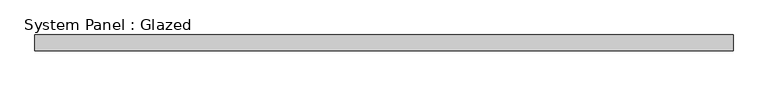
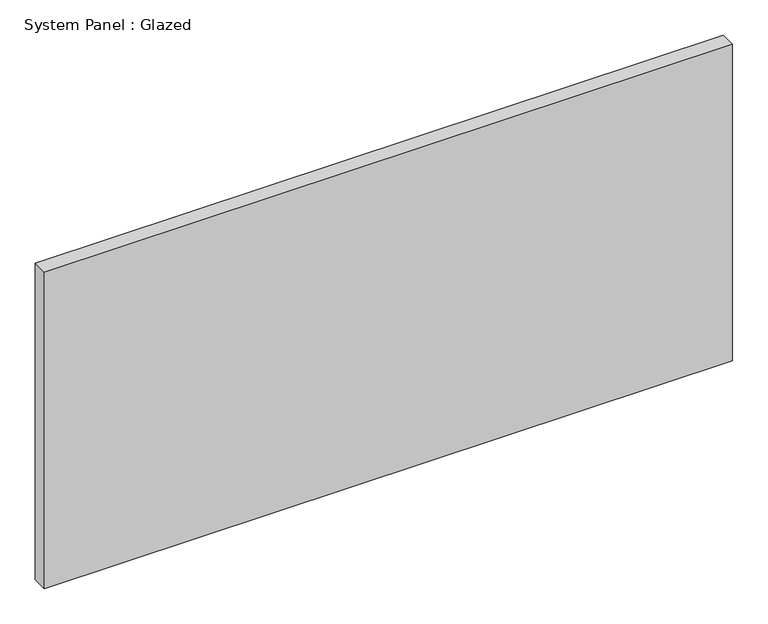
"""IFC4 building model written with IfcOpenShell, lengths in millimetres: plate geometry, System Panel : Glazed."""

from ifc_helpers import new_model, si_unit, origin, origin_with_axes, place, context, project, spatial, polyline, outline, extrude, source, transform, mapped, element, save


def system_panel_glazed_79634188(model_context):
    return source(origin(), model_context, "Body", "SweptSolid", [
        extrude(outline(polyline([(561.975, 19.05), (-561.975, 19.05), (-561.975, 44.45), (561.975, 44.45), (561.975, 19.05)])), origin_with_axes(), (0.0, 0.0, 1.0), 546.1),
    ])


if __name__ == "__main__":
    model = new_model("IFC4")
    model_context = context("Model", 3, world=origin())
    ifc_project = project(units=[si_unit("LENGTHUNIT", "METRE", prefix="MILLI")], contexts=[model_context])
    site = spatial("IfcSite", under=ifc_project)
    building = spatial("IfcBuilding", under=site)
    placement = place(None, origin())
    system_panel_glazed_shape = system_panel_glazed_79634188(model_context)
    element("IfcPlate", 1, ObjectType="System Panel : Glazed", at=placement, inside=building, context=model_context, shape_type="MappedRepresentation", body=[
        mapped(system_panel_glazed_shape, transform((0.0, 0.0, 0.0), x_axis=(1.0, 0.0, 0.0), y_axis=(0.0, 1.0, 0.0), z_axis=(0.0, 0.0, 1.0))),
    ])
    save(model, "model.ifc")

# Revit data of these elements
# Type "System Panel : Glazed"
#   Construction Type Id = "GSP4R"
#   Analytic Construction = "1/8 in Pilkington single glazing"
#   Visual Light Transmittance = 0.9
#   Solar Heat Gain Coefficient = 0.86
#   Heat Transfer Coefficient (U) = 1.18115 BTU/(h·ft²·°F)
# Element 1 (IfcPlate, "System Panel : Glazed")
#   Materials on its faces: "Glass"
# Materials
#   "Glass": class "Glass", colour RGB 0 128 192, transparency 0.75, Description = "Soda Lime Glass", Cost = 0
